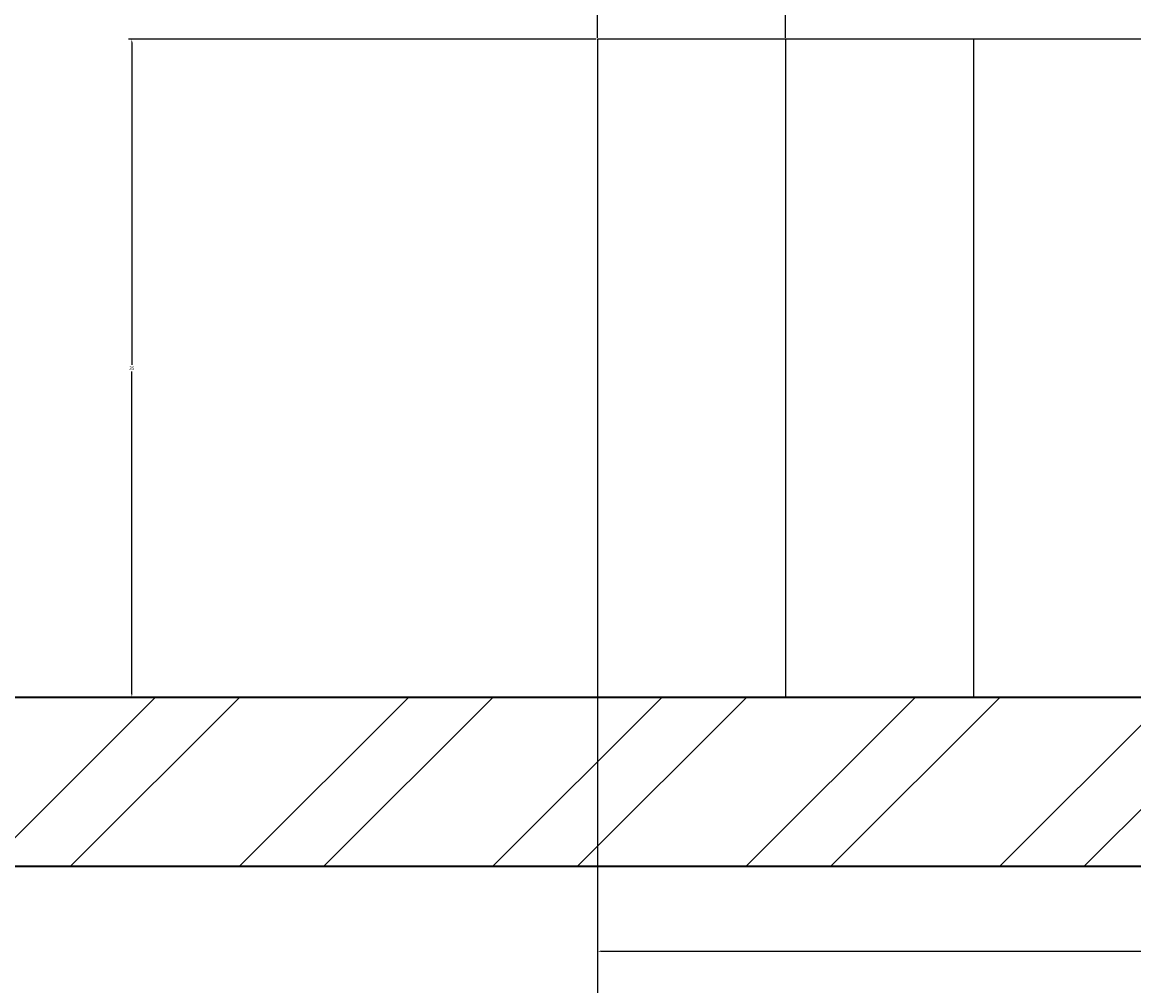
# Model space of a CAD drawing. Units: inches. Extents: x 2166 to 3588, y 1959 to 2628.
# Tile 6 of 13: x 3398 to 3457, y 2016 to 2067. Entities that reach past the tile are written whole.
import ezdxf

# ---------------------------------------------------------------- set-up
doc = ezdxf.new("R2010")
doc.units = ezdxf.units.IN
for name, color, linetype, lineweight in [('A-ANNO-DIMS', 2, 'Continuous', 18), ('A-WALL-PATT', 20, 'Continuous', 13), ('Staircase', 136, 'Continuous', 25), ('WALL', 40, 'Continuous', 35)]:
    doc.layers.add(name, color=color, linetype=linetype, lineweight=lineweight)
doc.styles.get("Standard").update_dxf_attribs({"font": 'arial.ttf'})
doc.dimstyles.get("Standard").update_dxf_attribs({"dimtxt": 0.18, "dimasz": 0.18, "dimexe": 0.18, "dimexo": 0.0625, "dimgap": 0.09, "dimtad": 0, "dimtih": 1, "dimtoh": 1, "dimdec": 4, "dimzin": 0, "dimdsep": 46, "dimtxsty": 'Standard', "dimcen": 0.09, "dimadec": 0, "dimazin": 0, "dimtfac": 1, "dimtdec": 4, "dimtofl": 0, "dimtmove": 0, "dimatfit": 3, "dimfxl": 1, "dimtolj": 1, "dimtzin": 0, "dimarcsym": 0})

# ---------------------------------------------------------------- blocks, each defined once
blk = doc.blocks.new('STAIR-RETURN-FLIGHTS')
for p, q in [((90, 35), (0, 35)), ((0, 35), (0, 0)), ((10, 35), (10, 0)), ((20, 35), (20, 0))]:
    blk.add_line(p, q)
blk = doc.blocks.new('*D17')
at = {"layer": 'A-ANNO-DIMS', "color": 0, "lineweight": -2, "transparency": 16777216}
for p, q in [((3428.471, 2030.916), (3428.471, 2017.299)), ((3518.471, 2030.916), (3518.471, 2017.299)), ((3428.651, 2017.479), (3472.538, 2017.479)), ((3518.291, 2017.479), (3474.403, 2017.479))]:
    blk.add_line(p, q, dxfattribs=at)
at = {"layer": 'A-ANNO-DIMS', "color": 0, "transparency": 16777216}
for points in [[(3428.651, 2017.509), (3428.651, 2017.449), (3428.471, 2017.479)], [(3518.291, 2017.509), (3518.291, 2017.449), (3518.471, 2017.479)]]:
    blk.add_solid(points, dxfattribs=at)
at = {"layer": 'Defpoints', "color": 0, "transparency": 16777216}
for p in [(3428.471, 2030.979), (3518.471, 2030.979), (3518.471, 2017.479)]:
    blk.add_point(p, dxfattribs=at)
at = {"layer": 'A-ANNO-DIMS', "color": 0, "transparency": 16777216, "insert": (3473.471, 2017.479), "char_height": 0.18, "attachment_point": 5}
blk.add_mtext('\\A1;STAIR 90 TYP.', dxfattribs=at)
blk = doc.blocks.new('*D50')
at = {"layer": 'A-ANNO-DIMS', "color": 0, "lineweight": -2, "transparency": 16777216}
for p, q in [((3236.471, 2030.916), (3236.471, 1997.049)), ((3428.471, 2030.916), (3428.471, 1997.049)), ((3236.651, 1997.229), (3332.191, 1997.229)), ((3428.291, 1997.229), (3332.75, 1997.229))]:
    blk.add_line(p, q, dxfattribs=at)
at = {"layer": 'A-ANNO-DIMS', "color": 0, "transparency": 16777216}
for points in [[(3236.651, 1997.259), (3236.651, 1997.199), (3236.471, 1997.229)], [(3428.291, 1997.259), (3428.291, 1997.199), (3428.471, 1997.229)]]:
    blk.add_solid(points, dxfattribs=at)
at = {"layer": 'Defpoints', "color": 0, "transparency": 16777216}
for p in [(3236.471, 2030.979), (3428.471, 2030.979), (3428.471, 1997.229)]:
    blk.add_point(p, dxfattribs=at)
at = {"layer": 'A-ANNO-DIMS', "color": 0, "transparency": 16777216, "insert": (3332.471, 1997.229), "char_height": 0.18, "attachment_point": 5}
blk.add_mtext('\\A1;192', dxfattribs=at)
blk = doc.blocks.new('*D53')
at = {"layer": 'A-ANNO-DIMS', "color": 0, "lineweight": -2, "transparency": 16777216}
for p, q in [((3428.471, 2066.041), (3428.471, 2454.909)), ((3428.651, 2454.729), (3433.26, 2454.729)), ((3438.291, 2454.729), (3433.681, 2454.729)), ((3438.471, 2066.041), (3438.471, 2454.909))]:
    blk.add_line(p, q, dxfattribs=at)
at = {"layer": 'A-ANNO-DIMS', "color": 0, "transparency": 16777216}
for points in [[(3428.651, 2454.759), (3428.651, 2454.699), (3428.471, 2454.729)], [(3438.291, 2454.759), (3438.291, 2454.699), (3438.471, 2454.729)]]:
    blk.add_solid(points, dxfattribs=at)
at = {"layer": 'Defpoints', "color": 0, "transparency": 16777216}
for p in [(3438.471, 2454.729), (3428.471, 2065.979), (3438.471, 2065.979)]:
    blk.add_point(p, dxfattribs=at)
at = {"layer": 'A-ANNO-DIMS', "color": 0, "transparency": 16777216, "insert": (3433.471, 2454.729), "char_height": 0.18, "attachment_point": 5}
blk.add_mtext('\\A1;10', dxfattribs=at)
blk = doc.blocks.new('*D54')
at = {"layer": 'A-ANNO-DIMS', "color": 0, "lineweight": -2, "transparency": 16777216}
for p, q in [((3428.408, 2065.979), (3403.541, 2065.979)), ((3403.721, 2065.799), (3403.721, 2048.661)), ((3403.721, 2031.159), (3403.721, 2048.297)), ((3428.408, 2030.979), (3403.541, 2030.979))]:
    blk.add_line(p, q, dxfattribs=at)
at = {"layer": 'A-ANNO-DIMS', "color": 0, "transparency": 16777216}
for points in [[(3403.691, 2065.799), (3403.751, 2065.799), (3403.721, 2065.979)], [(3403.691, 2031.159), (3403.751, 2031.159), (3403.721, 2030.979)]]:
    blk.add_solid(points, dxfattribs=at)
at = {"layer": 'Defpoints', "color": 0, "transparency": 16777216}
for p in [(3403.721, 2065.979), (3428.471, 2065.979), (3428.471, 2030.979)]:
    blk.add_point(p, dxfattribs=at)
at = {"layer": 'A-ANNO-DIMS', "color": 0, "transparency": 16777216, "insert": (3403.721, 2048.479), "char_height": 0.18, "attachment_point": 5}
blk.add_mtext('\\A1;35', dxfattribs=at)

msp = doc.modelspace()

# ---------------------------------------------------------------- hatches: boundary and pattern name
at = {"layer": 'A-WALL-PATT'}
h = msp.add_hatch(dxfattribs=at)
h.set_pattern_fill('ANSI32', color=256)
h.paths.add_polyline_path([(3563.471, 2429.979), (3227.471, 2429.979), (3227.471, 2021.979), (3563.471, 2021.979)])
h.paths.add_polyline_path([(3236.471, 2420.979), (3554.471, 2420.979), (3554.471, 2111.979), (3236.471, 2111.979)], flags=16)
h.paths.add_polyline_path([(3236.471, 2102.979), (3554.471, 2102.979), (3554.471, 2030.979), (3236.471, 2030.979)], flags=16)
h.paths.add_polyline_path([(3518.471, 2085.283), (3518.471, 2067.979), (3458.471, 2067.979), (3458.471, 2085.283)], flags=0)
h.paths.add_polyline_path([(3434.656, 2082.283), (3442.194, 2082.283), (3442.194, 2087.514), (3434.656, 2087.514)], flags=8)
h.paths.add_polyline_path([(3522.671, 2094.512), (3521.752, 2052.984), (3545.541, 2052.457), (3546.46, 2093.986)], flags=8)

# ---------------------------------------------------------------- linework, layer by layer
at = {"layer": 'WALL'}
msp.add_lwpolyline([(3227.471, 2429.979), (3563.471, 2429.979), (3563.471, 2021.979), (3227.471, 2021.979)], close=True, dxfattribs=at)
msp.add_lwpolyline([(3554.471, 2102.979), (3554.471, 2030.979), (3236.471, 2030.979), (3236.471, 2102.979)], dxfattribs=at)

# ---------------------------------------------------------------- block references
at = {"layer": 'Staircase'}
msp.add_blockref('STAIR-RETURN-FLIGHTS', (3428.471, 2030.979), dxfattribs=at)

# ---------------------------------------------------------------- dimensions: what is measured, and where the dimension line sits
at = {"layer": 'A-ANNO-DIMS'}
for base, p1, p2, picture, middle in [((3438.471, 2454.729), (3428.471, 2065.979), (3438.471, 2065.979), '*D53', (3433.471, 2454.729)), ((3428.471, 1997.229), (3236.471, 2030.979), (3428.471, 2030.979), '*D50', (3332.471, 1997.229))]:
    dim = msp.add_linear_dim(base=base, p1=p1, p2=p2, dimstyle='Standard', override={"dimdec": 0, "dimlfac": 1, "dimrnd": 0, "dimzin": 0, "dimdsep": 46, "dimlunit": 2}, dxfattribs=at)
    dim.commit()
    dim.dimension.update_dxf_attribs({"geometry": picture, "text_midpoint": middle})
dim = msp.add_linear_dim(base=(3403.721, 2065.979), p1=(3428.471, 2030.979), p2=(3428.471, 2065.979), angle=90, dimstyle='Standard', override={"dimdec": 0, "dimlfac": 1, "dimrnd": 0, "dimzin": 0, "dimdsep": 46, "dimlunit": 2}, dxfattribs=at)
dim.commit()
dim.dimension.update_dxf_attribs({"geometry": '*D54', "text_midpoint": (3403.721, 2048.479)})
dim = msp.add_linear_dim(base=(3518.471, 2017.479), p1=(3428.471, 2030.979), p2=(3518.471, 2030.979), text='STAIR <> TYP.', dimstyle='Standard', override={"dimdec": 0, "dimlfac": 1, "dimrnd": 0, "dimzin": 0, "dimdsep": 46, "dimlunit": 2}, dxfattribs=at)
dim.commit()
dim.dimension.update_dxf_attribs({"geometry": '*D17', "text_midpoint": (3473.471, 2017.479)})

doc.saveas('drawing.dxf')
